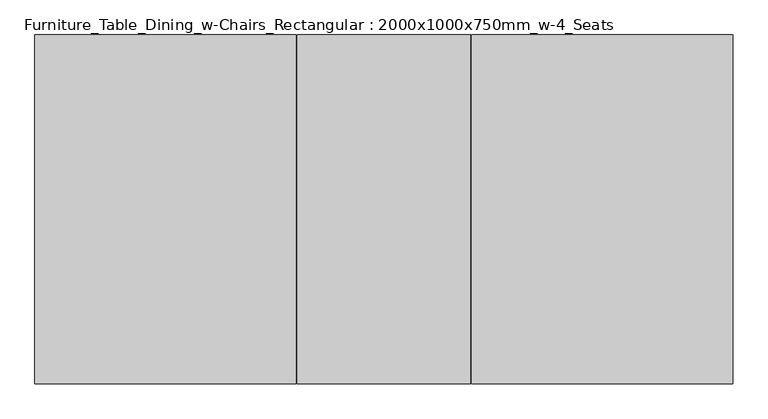
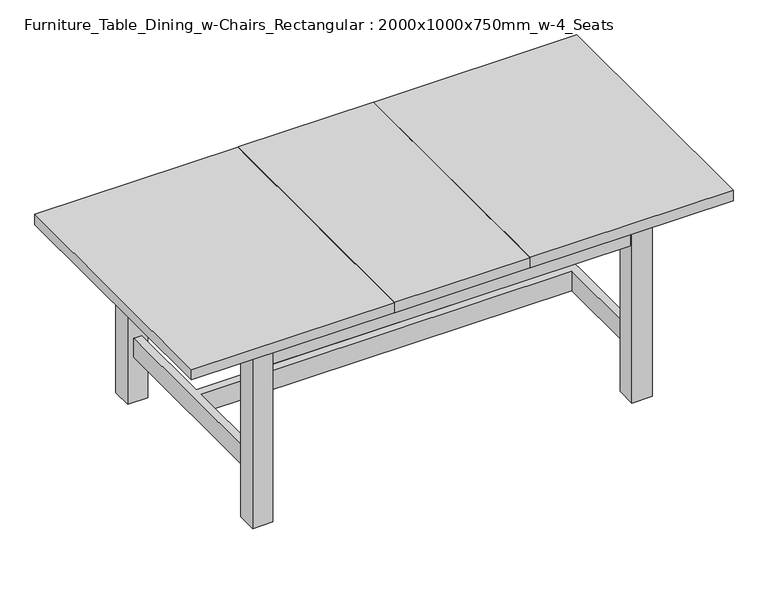
"""IFC4 building model written with IfcOpenShell, lengths in millimetres: furniture geometry, Furniture_Table_Dining_w-Chairs_Rectangular : 2000x1000x750mm_w-4_Seats."""

from ifc_helpers import new_model, si_unit, frame, origin, origin_with_axes, place, context, project, spatial, polyline, outline, extrude, faceted_brep, source, transform, mapped, element, save


def furniture_table_dining_w_chairs_rectangular_2000x1000x750mm_b8cbee69(model_context):
    return source(origin(), model_context, "Body", "SolidModel", [
        faceted_brep([(1118.1787219, -455.6453708, 750.0), (1118.1787219, 544.3546292, 750.0), (369.6787219, 544.3546292, 750.0), (369.6787219, -455.6453708, 750.0), (-881.8212781, 544.3546292, 750.0), (-881.8212781, -455.6453708, 750.0), (-133.3212781, -455.6453708, 750.0), (-133.3212781, 544.3546292, 750.0), (366.6787219, 544.3546292, 750.0), (-130.3212781, 544.3546292, 750.0), (-130.3212781, -455.6453708, 750.0), (366.6787219, -455.6453708, 750.0), (-881.8212781, -455.6453708, 710.0), (-881.8212781, 544.3546292, 710.0), (-133.3212781, 544.3546292, 710.0), (-131.8212781, 542.8546292, 710.0), (-130.3212781, 544.3546292, 710.0), (366.6787219, 544.3546292, 710.0), (368.1787219, 542.8546292, 710.0), (369.6787219, 544.3546292, 710.0), (1118.1787219, 544.3546292, 710.0), (1118.1787219, -455.6453708, 710.0), (369.6787219, -455.6453708, 710.0), (368.1787219, -454.1453708, 710.0), (366.6787219, -455.6453708, 710.0), (-130.3212781, -455.6453708, 710.0), (-131.8212781, -454.1453708, 710.0), (-133.3212781, -455.6453708, 710.0), (-131.8212781, 542.8546292, 748.5), (368.1787219, 542.8546292, 748.5), (-131.8212781, -454.1453708, 748.5), (368.1787219, -454.1453708, 748.5)], [[[0, 1, 2, 3]], [[4, 5, 6, 7]], [[8, 9, 10, 11]], [[12, 13, 14, 15, 16, 17, 18, 19, 20, 21, 22, 23, 24, 25, 26, 27]], [[1, 0, 21, 20]], [[9, 8, 17, 16]], [[1, 20, 19, 2]], [[13, 4, 7, 14]], [[5, 4, 13, 12]], [[11, 10, 25, 24]], [[21, 0, 3, 22]], [[5, 12, 27, 6]], [[15, 28, 9, 16]], [[28, 15, 14, 7]], [[18, 29, 2, 19]], [[29, 18, 17, 8]], [[9, 28, 30, 10]], [[28, 7, 6, 30]], [[2, 29, 31, 3]], [[29, 8, 11, 31]], [[10, 30, 26, 25]], [[30, 6, 27, 26]], [[3, 31, 23, 22]], [[31, 11, 24, 23]]]),
        extrude(outline(polyline([(-544.3212781, -393.1453708), (-619.3212781, -393.1453708), (-619.3212781, -318.1453708), (-544.3212781, -318.1453708), (-544.3212781, -393.1453708)])), origin_with_axes(), (0.0, 0.0, 1.0), 710.0),
        extrude(outline(polyline([(780.6787219, 481.8546292), (855.6787219, 481.8546292), (855.6787219, 406.8546292), (780.6787219, 406.8546292), (780.6787219, 481.8546292)])), origin_with_axes(), (0.0, 0.0, 1.0), 710.0),
        extrude(outline(polyline([(780.6787219, -318.1453708), (855.6787219, -318.1453708), (855.6787219, -393.1453708), (780.6787219, -393.1453708), (780.6787219, -318.1453708)])), origin_with_axes(), (0.0, 0.0, 1.0), 710.0),
        extrude(outline(polyline([(-544.3212781, 481.8546292), (-544.3212781, 406.8546292), (-619.3212781, 406.8546292), (-619.3212781, 481.8546292), (-544.3212781, 481.8546292)])), origin_with_axes(), (0.0, 0.0, 1.0), 710.0),
        extrude(outline(polyline([(-566.8212781, -318.1453708), (-596.8212781, -318.1453708), (-596.8212781, 406.8546292), (-566.8212781, 406.8546292), (-566.8212781, 59.3546292), (803.1787219, 59.3546292), (803.1787219, 406.8546292), (833.1787219, 406.8546292), (833.1787219, -318.1453708), (803.1787219, -318.1453708), (803.1787219, 29.3546292), (-566.8212781, 29.3546292), (-566.8212781, -318.1453708)])), frame((0.0, 0.0, 175.0), z_axis=(0.0, 0.0, 1.0), x_axis=(1.0, 0.0, 0.0)), (0.0, 0.0, 1.0), 75.0),
        extrude(outline(polyline([(-544.3212781, 474.3546292), (780.6787219, 474.3546292), (780.6787219, 454.3546292), (-544.3212781, 454.3546292), (-544.3212781, 474.3546292)])), frame((0.0, 0.0, 610.0), z_axis=(0.0, 0.0, 1.0), x_axis=(1.0, 0.0, 0.0)), (0.0, 0.0, 1.0), 100.0),
        extrude(outline(polyline([(-611.8212781, -318.1453708), (-611.8212781, 406.8546292), (-591.8212781, 406.8546292), (-591.8212781, -318.1453708), (-611.8212781, -318.1453708)])), frame((0.0, 0.0, 610.0), z_axis=(0.0, 0.0, 1.0), x_axis=(1.0, 0.0, 0.0)), (0.0, 0.0, 1.0), 100.0),
        extrude(outline(polyline([(780.6787219, -385.6453708), (-544.3212781, -385.6453708), (-544.3212781, -365.6453708), (780.6787219, -365.6453708), (780.6787219, -385.6453708)])), frame((0.0, 0.0, 610.0), z_axis=(0.0, 0.0, 1.0), x_axis=(1.0, 0.0, 0.0)), (0.0, 0.0, 1.0), 100.0),
        extrude(outline(polyline([(848.1787219, 406.8546292), (848.1787219, -318.1453708), (828.1787219, -318.1453708), (828.1787219, 406.8546292), (848.1787219, 406.8546292)])), frame((0.0, 0.0, 610.0), z_axis=(0.0, 0.0, 1.0), x_axis=(1.0, 0.0, 0.0)), (0.0, 0.0, 1.0), 100.0),
    ])


if __name__ == "__main__":
    model = new_model("IFC4")
    model_context = context("Model", 3, world=origin())
    ifc_project = project(units=[si_unit("LENGTHUNIT", "METRE", prefix="MILLI")], contexts=[model_context])
    site = spatial("IfcSite", under=ifc_project)
    building = spatial("IfcBuilding", under=site)
    placement = place(None, origin())
    furniture_table_dining_w_chairs_rectangular_2000x1000x750mm_shape = furniture_table_dining_w_chairs_rectangular_2000x1000x750mm_b8cbee69(model_context)
    element("IfcFurniture", 1, ObjectType="Furniture_Table_Dining_w-Chairs_Rectangular : 2000x1000x750mm_w-4_Seats", at=placement, inside=building, context=model_context, shape_type="MappedRepresentation", body=[
        mapped(furniture_table_dining_w_chairs_rectangular_2000x1000x750mm_shape, transform((0.0, 0.0, 0.0), x_axis=(1.0, 0.0, 0.0), y_axis=(0.0, 1.0, 0.0), z_axis=(0.0, 0.0, 1.0))),
    ])
    save(model, "model.ifc")

# Revit data of these elements
# Type "Furniture_Table_Dining_w-Chairs_Rectangular : 2000x1000x750mm_w-4_Seats"
#   Keynote = "N"
#   Width = 3' - 3.37008"
#   Table Top Thickness = 0' - 1.5748"
#   Table Height = 2' - 5.52756"
#   Length = 6' - 6.74016"
#   Leg Width = 0' - 2.95276"
#   Leg Spacing Width = 2' - 7.49606"
#   Leg Spacing Length = 4' - 7.11811"
#   Chair Side Spacing = 2' - 3.55906"
#   Centre Piece = 1' - 7.68504"
#   Vis - End Chairs = no
#   Material Table = Wood - Birch
#   Material Chair Structure = Wood - Birch
#   Material Chair Covering = Fabric - Beige
#   Default Elevation = 0
# Element 1 (IfcFurniture, "Furniture_Table_Dining_w-Chairs_Rectangular : 2000x1000x750mm_w-4_Seats")
#   Materials on its faces: "Wood - Birch"
# Materials
#   "Wood - Birch": class "Wood", colour RGB 213 164 103, transparency 0
#   "Fabric - Beige": class "Fabric", colour RGB 231 227 195, transparency 0
